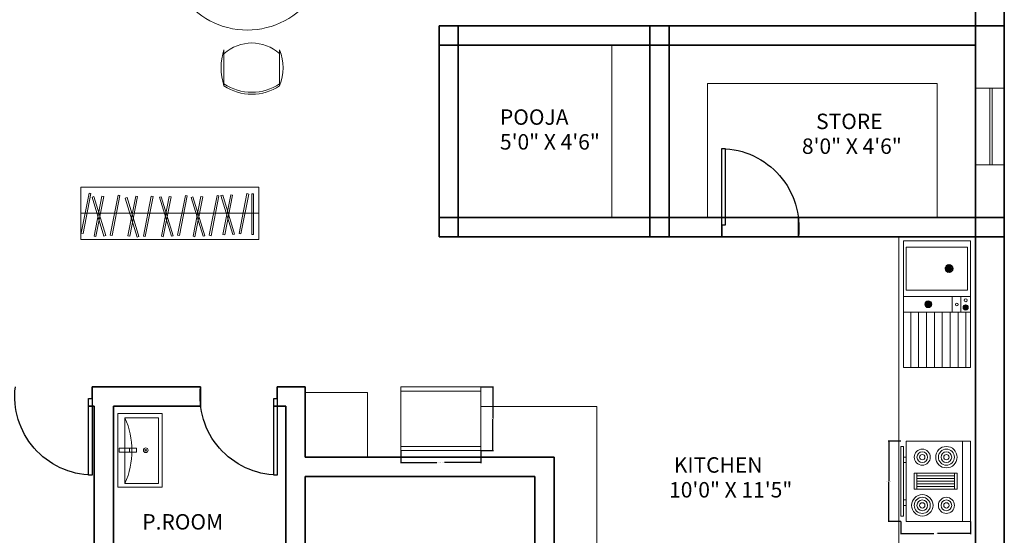
# Model space of a CAD drawing. Units: inches. Extents: x -61 to 1599, y -1316 to 257.
# Tile 168 of 204: x 1214 to 1523, y -1099 to -937. Entities that reach past the tile are written whole.
import ezdxf

# ---------------------------------------------------------------- set-up
doc = ezdxf.new("R2010")
doc.units = ezdxf.units.IN
doc.header["$MEASUREMENT"] = 0
doc.linetypes.add('ACAD_ISO02W100', pattern=[15, 12, -3])
for name, color, linetype, lineweight in [('A-ANNO-DIMS', 2, 'Continuous', 18), ('A-AREA-IDEN', 1, 'Continuous', 18), ('A-EQPM', 9, 'Continuous', 18), ('A-FLOR-CASE', 8, 'Continuous', 18), ('A-FLOR-FIXT', 8, 'Continuous', 18), ('A-WALL-JAMB', 4, 'ACAD_ISO02W100', 25), ('DOORS', 2, 'Continuous', 25), ('FURNITURE', 83, 'Continuous', 18), ('WALLS', 4, 'Continuous', 35), ('WINDOWS', 220, 'Continuous', 18)]:
    doc.layers.add(name, color=color, linetype=linetype, lineweight=lineweight)
doc.layers.add('FUR', color=83, linetype='Continuous')
doc.styles.get("Standard").update_dxf_attribs({"font": 'arial.ttf'})
doc.dimstyles.get("Standard").update_dxf_attribs({"dimtxt": 0.18, "dimasz": 0.18, "dimexe": 0.18, "dimexo": 0.0625, "dimgap": 0.09, "dimtad": 0, "dimtih": 1, "dimtoh": 1, "dimdec": 0, "dimzin": 0, "dimdsep": 46, "dimlunit": 3, "dimtxsty": 'Standard', "dimcen": 0.09, "dimadec": 0, "dimazin": 0, "dimtfac": 1, "dimtdec": 0, "dimtofl": 0, "dimtmove": 0, "dimatfit": 3, "dimfxl": 1, "dimtolj": 1, "dimtzin": 0, "dimarcsym": 0})

# ---------------------------------------------------------------- blocks, each defined once
blk = doc.blocks.new('Range-Oven - 30 in top')
for p, q in [((0, -3), (30, -3)), ((12, -6), (18, -6)), ((13, -20), (13, -6)), ((14, -6), (14, -20)), ((15, -20), (15, -6)), ((16, -6), (16, -20)), ((17, -20), (17, -6)), ((18, -20), (12, -20)), ((6, -24), (6, -25)), ((8, -25), (8, -24)), ((22, -25), (22, -24)), ((24, -24), (24, -25))]:
    blk.add_line(p, q)
for points in [[(0, -24), (0, 0), (30, 0), (30, -24)], [(12, -21), (12, -5), (18, -5), (18, -21)], [(2, -26), (2, -25), (28, -25), (28, -26)]]:
    blk.add_lwpolyline(points, close=True)
for centre, radius in [((6, -9), 4), ((6, -9), 3), ((6, -9), 2), ((24, -9), 3), ((24, -9), 2), ((6, -9), 1), ((24, -9), 1), ((24, -18), 4), ((6, -18), 3), ((6, -18), 2), ((6, -18), 1), ((24, -18), 3), ((24, -18), 2), ((24, -18), 1)]:
    blk.add_circle(centre, radius)
blk = doc.blocks.new('DOOR-SWING-24')
blk.add_line((0, 0), (0, 3.6))
blk.add_lwpolyline([(0, 0), (0, -24), (1.05, -24), (1.05, 0)], close=True)
blk.add_arc((-0.44, 0.62), 24.62, 271.0259, 6.9559)
blk = doc.blocks.new('WIN-24IN')
for p, q in [((0, 4.5), (0, 9)), ((0, 9), (0, 0)), ((24, 9), (24, 0)), ((0, 5.19), (24, 5.19)), ((0, 4.5), (24, 4.5))]:
    blk.add_line(p, q)
blk = doc.blocks.new('LAVATORY-WALL-2')
blk.add_line((3.67, 10.96), (3.67, 12.19))
for points in [[(0, 23.07), (13.87, 23.07), (13.87, 0), (0, 0)], [(12.66, 21.73), (12.66, 1.19), (2.2, 1.19), (2.2, 21.73)], [(5.78, 12.19), (5.78, 10.96), (0.4, 10.96), (0.4, 12.19)]]:
    blk.add_lwpolyline(points, close=True)
for radius in [0.74, 0.233]:
    blk.add_circle((8.7, 11.57), radius)
blk.add_arc((-20.86, 11.46), 25.25, 335.9939, 24.0061)
blk = doc.blocks.new('*U268')
at = {"layer": 'FUR'}
blk.add_line((0.41, 1.36), (0.41, 0.68), dxfattribs=at)
blk.add_open_spline([(0.41, 1.36), (0.24, 1.25), (-0.09, 1.02), (0.41, 0.7), (0.83, 0.34), (0.55, 0.11), (0.41, 0)], degree=3, knots=[0, 0, 0, 0, 0.474547, 0.949094, 1.393355, 1.837616, 1.837616, 1.837616, 1.837616], dxfattribs=at)
blk = doc.blocks.new('*U269')
at = {"layer": 'FUR', "transparency": 16777216}
for p, rotation in [((531.82, -257.55), 308.5714285714286), ((532.89, -258.18), 51.42857142857144), ((532.03, -256.89), 257.1428571428571), ((533.36, -257.68), 102.8571428571428), ((532.68, -256.65), 205.7142857142857), ((533.27, -257), 154.2857142857143)]:
    blk.add_blockref('*U268', p, dxfattribs=dict(at, rotation=rotation))
blk.add_blockref('*U268', (532.2, -258.12), dxfattribs=at)
blk = doc.blocks.new('*U270')
at = {"layer": 'FUR'}
blk.add_line((0.74, 2.46), (0.74, 1.23), dxfattribs=at)
blk.add_open_spline([(0.74, 2.46), (0.44, 2.26), (-0.16, 1.84), (0.74, 1.26), (1.5, 0.61), (0.99, 0.2), (0.74, 0)], degree=3, knots=[0, 0, 0, 0, 0.85637, 1.712739, 2.514455, 3.316171, 3.316171, 3.316171, 3.316171], dxfattribs=at)
blk = doc.blocks.new('*U271')
at = {"layer": 'FUR', "transparency": 16777216}
for p, rotation in [((959.72, -464.77), 308.5714285714286), ((961.65, -465.92), 51.42857142857144), ((960.11, -463.59), 257.1428571428571), ((962.51, -465.02), 102.8571428571428), ((961.27, -463.15), 205.7142857142858), ((962.34, -463.79), 154.2857142857143)]:
    blk.add_blockref('*U270', p, dxfattribs=dict(at, rotation=rotation))
blk.add_blockref('*U270', (960.41, -465.81), dxfattribs=at)
blk = doc.blocks.new('*U266')
at = {"layer": 'FUR'}
blk.add_line((0.41, 1.36), (0.41, 0.68), dxfattribs=at)
blk.add_open_spline([(0.41, 1.36), (0.24, 1.25), (-0.09, 1.02), (0.41, 0.7), (0.83, 0.34), (0.55, 0.11), (0.41, 0)], degree=3, knots=[0, 0, 0, 0, 0.474547, 0.949094, 1.393355, 1.837616, 1.837616, 1.837616, 1.837616], dxfattribs=at)
blk = doc.blocks.new('*U267')
at = {"layer": 'FUR', "transparency": 16777216}
for p, rotation in [((531.82, -257.55), 308.5714285714286), ((532.89, -258.18), 51.42857142857144), ((532.03, -256.89), 257.1428571428571), ((533.36, -257.68), 102.8571428571428), ((532.68, -256.65), 205.7142857142857), ((533.27, -257), 154.2857142857143)]:
    blk.add_blockref('*U266', p, dxfattribs=dict(at, rotation=rotation))
blk.add_blockref('*U266', (532.2, -258.12), dxfattribs=at)
blk = doc.blocks.new('SINK-WITH-DRAINBOARD')
for p, q in [((14.29, 30.97), (14.29, 29.74)), ((0, 22.17), (20.98, 22.17)), ((15.24, 17.27), (15.24, 22.17)), ((17.97, 22.17), (17.97, 17.27)), ((7.79, 19.82), (7.79, 19.14)), ((19.48, 18.8), (19.48, 18.12)), ((0, 17.27), (20.98, 17.27)), ((2.27, 0), (2.27, 17.27)), ((4.74, 0), (4.74, 17.27)), ((7.21, 0), (7.21, 17.27)), ((9.69, 0), (9.69, 17.27)), ((12.16, 0), (12.16, 17.27)), ((14.63, 0), (14.63, 17.27)), ((17.1, 0), (17.1, 17.27)), ((19.58, 0), (19.58, 17.27))]:
    blk.add_line(p, q)
for points in [[(20.98, 0), (0, 0), (0, 39.63), (20.98, 39.63)], [(20.07, 24.22), (0.86, 24.22), (0.86, 37.7), (20.07, 37.7)]]:
    blk.add_lwpolyline(points, close=True)
for centre, radius in [((14.29, 30.97), 1.23), ((7.78, 19.81), 1.08), ((7.78, 19.81), 0.877), ((7.79, 19.82), 0.682), ((16.69, 19.72), 0.419), ((19.48, 18.8), 0.816), ((19.48, 18.8), 0.816), ((19.48, 18.8), 0.682), ((19.48, 21.05), 0.455)]:
    blk.add_circle(centre, radius)
for name, p in [('*U271', (-946.85, 495.54)), ('*U269', (-524.82, 277.26)), ('*U267', (-513.12, 276.24))]:
    blk.add_blockref(name, p)
blk = doc.blocks.new('KITCHEN-BASE-UNIT')
for p, q in [((25.07, 18.6), (0, 18.6)), ((25.07, 1.23), (0, 1.23))]:
    blk.add_line(p, q)
blk.add_lwpolyline([(25.07, 0), (0, 0), (0, 19.92), (25.07, 19.92)], close=True)
blk = doc.blocks.new('STORE-SHELVING')
for p, q in [((0, 42), (72, 42)), ((0, 12), (0, 42)), ((72, 42), (72, 12)), ((0, 0), (0, 12)), ((72, 0), (72, 12))]:
    blk.add_line(p, q)
blk = doc.blocks.new('DINING-TABLE-OVAL')
for p, q in [((20.06, 34.26), (38.12, 65.35)), ((20.69, 45.86), (30.12, 61.18)), ((27.51, 37.68), (36.94, 53.01))]:
    blk.add_line(p, q)
for centre, radius, start, end in [((28.99, 70.07), 25.36, 35.5172, 144.4828), ((85.79, 47.89), 85.79, 154.5151, 205.4849), ((-21.85, 47.89), 80.45, 332.689, 27.311), ((28.99, 24.89), 24.89, 213.9753, 326.0247)]:
    blk.add_arc(centre, radius, start, end)
blk = doc.blocks.new('DINING-CHAIR')
for p, q in [((0.9, 2.16), (0.9, 13.35)), ((18.35, 2.16), (18.35, 13.35))]:
    blk.add_line(p, q)
for centre, radius, start, end in [((9.63, 0.52), 15.52, 55.8098, 124.1902), ((17.78, 7.76), 17.78, 161.6455, 198.3545), ((9.63, -0.1), 15.52, 55.8098, 124.1902), ((4.51, 7.76), 14.92, 337.9646, 22.0354), ((9.63, 12.87), 12.87, 227.332, 312.668)]:
    blk.add_arc(centre, radius, start, end)
blk = doc.blocks.new('WARDROBE-HANGING-2')
blk.add_line((55.7, 8.23), (0, 8.23))
for points in [[(55.7, 16.46), (55.7, 0), (0, 0), (0, 16.46)], [(0.12, 2.03), (2.58, 14.54), (3.16, 14.43), (0.7, 1.92)], [(7.24, 1.1), (3.5, 13.29), (4.06, 13.46), (7.8, 1.28)], [(4.13, 1.08), (6.59, 13.59), (7.17, 13.48), (4.71, 0.97)], [(9.19, 1.4), (11.65, 13.91), (12.23, 13.8), (9.77, 1.29)], [(17.64, 0.82), (13.9, 13), (14.46, 13.18), (18.2, 0.99)], [(14.73, 1.14), (17.19, 13.65), (17.77, 13.54), (15.31, 1.03)], [(19.59, 1.12), (22.05, 13.62), (22.63, 13.51), (20.17, 1)], [(28.34, 1.05), (24.59, 13.24), (25.16, 13.41), (28.9, 1.22)], [(25.23, 1.03), (27.69, 13.54), (28.27, 13.43), (25.81, 0.92)], [(30.28, 1.35), (32.74, 13.86), (33.32, 13.75), (30.86, 1.24)], [(38.26, 1.05), (34.51, 13.23), (35.08, 13.41), (38.82, 1.22)], [(35.15, 1.03), (37.61, 13.54), (38.19, 13.42), (35.73, 0.92)], [(40.2, 1.35), (42.66, 13.86), (43.24, 13.74), (40.78, 1.23)], [(47.6, 1.58), (43.86, 13.76), (44.42, 13.94), (48.16, 1.75)], [(44.49, 1.56), (46.95, 14.07), (47.53, 13.95), (45.07, 1.45)], [(49.55, 1.88), (52.01, 14.39), (52.59, 14.27), (50.13, 1.77)], [(54.1, 14.33), (54.1, 1.58), (53.51, 1.58), (53.51, 14.33)]]:
    blk.add_lwpolyline(points, close=True)
blk = doc.blocks.new('*D638')
at = {"layer": 'A-ANNO-DIMS', "color": 0, "lineweight": -2, "transparency": 16777216}
for p, q in [((1490.26, -1069.14), (1486.37, -1069.14)), ((1486.55, -1069.32), (1486.55, -1081.53)), ((1486.55, -1094.1), (1486.55, -1081.89)), ((1490.26, -1094.28), (1486.37, -1094.28))]:
    blk.add_line(p, q, dxfattribs=at)
at = {"layer": 'A-ANNO-DIMS', "color": 0, "transparency": 16777216}
for points in [[(1486.52, -1069.32), (1486.58, -1069.32), (1486.55, -1069.14)], [(1486.52, -1094.1), (1486.58, -1094.1), (1486.55, -1094.28)]]:
    blk.add_solid(points, dxfattribs=at)
at = {"layer": 'DEFPOINTS', "color": 0, "transparency": 16777216}
for p in [(1490.32, -1069.14), (1486.55, -1094.28), (1490.32, -1094.28)]:
    blk.add_point(p, dxfattribs=at)
at = {"layer": 'A-ANNO-DIMS', "color": 0, "transparency": 16777216, "insert": (1486.55, -1081.71), "char_height": 0.18, "attachment_point": 5}
blk.add_mtext('\\A1;RANGE 25 TYP.', dxfattribs=at)
blk = doc.blocks.new('*D639')
at = {"layer": 'A-ANNO-DIMS', "color": 0, "lineweight": -2, "transparency": 16777216}
for p, q in [((1490.32, -1094.34), (1490.32, -1098.23)), ((1512.1, -1094.34), (1512.1, -1098.23)), ((1490.5, -1098.05), (1500.68, -1098.05)), ((1511.92, -1098.05), (1501.74, -1098.05))]:
    blk.add_line(p, q, dxfattribs=at)
at = {"layer": 'A-ANNO-DIMS', "color": 0, "transparency": 16777216}
for points in [[(1490.5, -1098.02), (1490.5, -1098.08), (1490.32, -1098.05)], [(1511.92, -1098.02), (1511.92, -1098.08), (1512.1, -1098.05)]]:
    blk.add_solid(points, dxfattribs=at)
at = {"layer": 'DEFPOINTS', "color": 0, "transparency": 16777216}
for p in [(1490.32, -1094.28), (1512.1, -1094.28), (1512.1, -1098.05)]:
    blk.add_point(p, dxfattribs=at)
at = {"layer": 'A-ANNO-DIMS', "color": 0, "transparency": 16777216, "insert": (1501.21, -1098.05), "char_height": 0.18, "attachment_point": 5}
blk.add_mtext('\\A1;22 TYP.', dxfattribs=at)
blk = doc.blocks.new('*D660')
at = {"layer": 'A-ANNO-DIMS', "color": 0, "lineweight": -2, "transparency": 16777216}
for p, q in [((1333.67, -1072.15), (1333.67, -1076.03)), ((1358.75, -1072.15), (1358.75, -1076.03)), ((1333.85, -1075.85), (1344.99, -1075.85)), ((1358.57, -1075.85), (1347.43, -1075.85))]:
    blk.add_line(p, q, dxfattribs=at)
at = {"layer": 'A-ANNO-DIMS', "color": 0, "transparency": 16777216}
for points in [[(1333.85, -1075.82), (1333.85, -1075.88), (1333.67, -1075.85)], [(1358.57, -1075.82), (1358.57, -1075.88), (1358.75, -1075.85)]]:
    blk.add_solid(points, dxfattribs=at)
at = {"layer": 'DEFPOINTS', "color": 0, "transparency": 16777216}
for p in [(1333.67, -1072.09), (1358.75, -1072.09), (1358.75, -1075.85)]:
    blk.add_point(p, dxfattribs=at)
at = {"layer": 'A-ANNO-DIMS', "color": 0, "transparency": 16777216, "insert": (1346.21, -1075.85), "char_height": 0.18, "attachment_point": 5}
blk.add_mtext('\\A1;BASE UNIT 25 TYP.', dxfattribs=at)
blk = doc.blocks.new('*D661')
at = {"layer": 'A-ANNO-DIMS', "color": 0, "lineweight": -2, "transparency": 16777216}
for p, q in [((1358.81, -1052.17), (1362.69, -1052.17)), ((1362.51, -1052.35), (1362.51, -1061.95)), ((1362.51, -1071.91), (1362.51, -1062.31)), ((1358.81, -1072.09), (1362.69, -1072.09))]:
    blk.add_line(p, q, dxfattribs=at)
at = {"layer": 'A-ANNO-DIMS', "color": 0, "transparency": 16777216}
for points in [[(1362.48, -1052.35), (1362.54, -1052.35), (1362.51, -1052.17)], [(1362.48, -1071.91), (1362.54, -1071.91), (1362.51, -1072.09)]]:
    blk.add_solid(points, dxfattribs=at)
at = {"layer": 'DEFPOINTS', "color": 0, "transparency": 16777216}
for p in [(1358.75, -1052.17), (1362.51, -1052.17), (1358.75, -1072.09)]:
    blk.add_point(p, dxfattribs=at)
at = {"layer": 'A-ANNO-DIMS', "color": 0, "transparency": 16777216, "insert": (1362.51, -1062.13), "char_height": 0.18, "attachment_point": 5}
blk.add_mtext('\\A1;20 TYP.', dxfattribs=at)

msp = doc.modelspace()

# ---------------------------------------------------------------- linework, layer by layer
at = {"layer": 'A-FLOR-CASE'}
for p, q in [((1489.7028, -1005.169), (1489.7028, -1029.169)), ((1489.7028, -1118.169), (1489.7028, -1029.169)), ((1358.7476, -1058.2566), (1395.0519, -1058.2566)), ((1395.0519, -1058.2566), (1395.0519, -1142.169))]:
    msp.add_line(p, q, dxfattribs=at)
for points in [[(1411.7028, -999.169), (1399.7505, -999.169), (1399.7505, -945.169), (1411.7028, -945.169)], [(1323.3268, -1074.169), (1303.7028, -1074.169), (1303.7028, -1053.915), (1323.3268, -1053.915)]]:
    msp.add_lwpolyline(points, close=True, dxfattribs=at)
at = {"layer": 'A-WALL-JAMB'}
for p, q in [((1434.2028, -1005.169), (1434.2028, -999.169)), ((1458.2028, -1005.169), (1458.1983, -999.169)), ((1236.999, -1052.169), (1236.999, -1058.169)), ((1271.017, -1052.169), (1271.017, -1058.169)), ((1295.017, -1052.169), (1295.017, -1058.169))]:
    msp.add_line(p, q, dxfattribs=at)
at = {"layer": 'WALLS'}
for p, q in [((1513.7028, -783.169), (1513.7028, -945.169)), ((1522.7028, -1211.169), (1522.7028, -837.0151)), ((1345.7028, -939.169), (1381.7028, -939.169)), ((1345.7028, -1005.169), (1345.7028, -939.169)), ((1351.7028, -1005.169), (1351.7028, -939.169)), ((1375.7028, -939.169), (1522.7028, -939.169)), ((1411.7028, -1005.169), (1411.7028, -939.169)), ((1417.7028, -1005.169), (1417.7028, -939.169)), ((1345.7028, -945.169), (1351.7028, -945.169)), ((1351.7028, -945.169), (1411.7028, -945.169)), ((1411.7028, -945.169), (1417.7028, -945.169)), ((1417.7028, -945.169), (1513.7028, -945.169)), ((1513.7028, -1052.169), (1513.7028, -945.169)), ((1345.7028, -999.169), (1522.7028, -999.169)), ((1411.7028, -999.169), (1522.7028, -999.169)), ((1345.7028, -1005.169), (1522.7028, -1005.169)), ((1411.7028, -1005.169), (1522.7028, -1005.169)), ((1236.999, -1052.169), (1271.017, -1052.169)), ((1295.017, -1052.169), (1303.7028, -1052.169)), ((1303.7028, -1052.169), (1303.7028, -1074.169)), ((1513.7028, -1052.169), (1513.7028, -1148.169)), ((1235.949, -1058.169), (1237.7028, -1058.169)), ((1237.7028, -1058.169), (1237.7028, -1202.169)), ((1243.7028, -1058.169), (1243.7028, -1137.169)), ((1243.7028, -1058.169), (1271.0214, -1058.169)), ((1293.967, -1058.169), (1297.7028, -1058.169)), ((1297.7028, -1058.169), (1297.7028, -1137.169)), ((1303.7028, -1074.169), (1381.7028, -1074.169)), ((1381.7028, -1074.169), (1381.7028, -1142.169)), ((1303.7028, -1080.169), (1303.7028, -1146.0672)), ((1303.7028, -1080.169), (1375.7028, -1080.169)), ((1375.7028, -1080.169), (1375.7028, -1174.9919))]:
    msp.add_line(p, q, dxfattribs=at)

# ---------------------------------------------------------------- block references
at = {"layer": 'A-EQPM', "xscale": 0.8378013827109642, "yscale": 0.8378013827109642, "zscale": 0.8378013827109642, "rotation": 270}
msp.add_blockref('Range-Oven - 30 in top', (1512.1022, -1069.1411), dxfattribs=at)
at = {"layer": 'A-FLOR-CASE'}
for name, p in [('STORE-SHELVING', (1429.703, -999.1691)), ('WARDROBE-HANGING-2', (1233.5089, -1006.0714)), ('KITCHEN-BASE-UNIT', (1333.674, -1072.0911))]:
    msp.add_blockref(name, p, dxfattribs=at)
at = {"layer": 'A-FLOR-FIXT'}
for name, p in [('SINK-WITH-DRAINBOARD', (1491.125, -1046.0901)), ('LAVATORY-WALL-2', (1245.1172, -1083.5756))]:
    msp.add_blockref(name, p, dxfattribs=at)
at = {"layer": 'DOORS', "extrusion": (0, 0, -1), "zscale": -1, "rotation": 180}
msp.add_blockref('DOOR-SWING-24', (-1434.2028, -1001.569), dxfattribs=at)
at = {"layer": 'DOORS', "extrusion": (0, 0, -1), "zscale": -1}
for p in [(-1236.999, -1055.769), (-1295.017, -1055.769)]:
    msp.add_blockref('DOOR-SWING-24', p, dxfattribs=at)
at = {"layer": 'FURNITURE'}
msp.add_blockref('DINING-TABLE-OVAL', (1256.634, -940.4721), dxfattribs=at)
at = {"layer": 'FURNITURE', "extrusion": (0, 0, -1), "zscale": -1, "rotation": 180}
msp.add_blockref('DINING-CHAIR', (-1277.4166, -944.5239), dxfattribs=at)
at = {"layer": 'WINDOWS', "rotation": 270}
msp.add_blockref('WIN-24IN', (1513.7027, -958.6117), dxfattribs=at)

# ---------------------------------------------------------------- texts
at = {"layer": 'A-AREA-IDEN'}
for s, height, p in [('POOJA', 4.8321, (1364.7531, -970.1266)), ('   STORE', 4.8321, (1459.3179, -971.4724)), ('5\'0" X 4\'6"', 4.832098, (1364.7531, -977.889)), ('8\'0" X 4\'6"', 4.832098, (1459.3179, -979.2347)), (' KITCHEN', 4.8321, (1417.7144, -1079.0292)), ('10\'0" X 11\'5"', 4.832098, (1417.7144, -1086.7915)), ('P.ROOM', 4.8321, (1252.7407, -1096.8233))]:
    msp.add_text(s, height=height, dxfattribs=at).set_placement(p)

# ---------------------------------------------------------------- dimensions: what is measured, and where the dimension line sits
at = {"layer": 'A-ANNO-DIMS'}
for base, p1, p2, angle, text, picture, middle in [((1362.5086, -1052.169), (1358.7476, -1072.0916), (1358.7476, -1052.169), 90, '<> TYP.', '*D661', (1362.5086, -1062.1303)), ((1486.5493, -1094.2751), (1490.3194, -1069.1411), (1490.3194, -1094.2751), 270, 'RANGE <> TYP.', '*D638', (1486.5493, -1081.7081))]:
    dim = msp.add_linear_dim(base=base, p1=p1, p2=p2, angle=angle, text=text, dimstyle='Standard', override={"dimdec": 0, "dimlfac": 1, "dimrnd": 0, "dimzin": 0, "dimdsep": 46, "dimlunit": 2}, dxfattribs=at)
    dim.commit()
    dim.dimension.update_dxf_attribs({"geometry": picture, "text_midpoint": middle})
for base, p1, p2, text, picture, middle in [((1358.7476, -1075.8526), (1333.6745, -1072.0916), (1358.7476, -1072.0916), 'BASE UNIT <> TYP.', '*D660', (1346.211, -1075.8526)), ((1512.1022, -1098.0452), (1490.3194, -1094.2751), (1512.1022, -1094.2751), '<> TYP.', '*D639', (1501.2108, -1098.0452))]:
    dim = msp.add_linear_dim(base=base, p1=p1, p2=p2, text=text, dimstyle='Standard', override={"dimdec": 0, "dimlfac": 1, "dimrnd": 0, "dimzin": 0, "dimdsep": 46, "dimlunit": 2}, dxfattribs=at)
    dim.commit()
    dim.dimension.update_dxf_attribs({"geometry": picture, "text_midpoint": middle})

doc.saveas('drawing.dxf')
